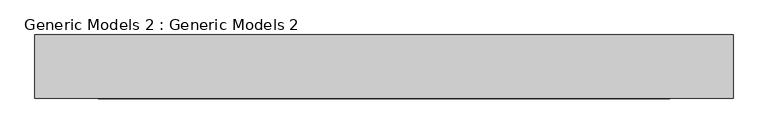
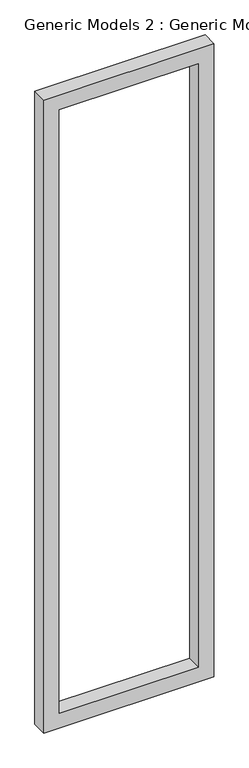
"""IFC4 building model written with IfcOpenShell, lengths in millimetres: proxy geometry, Generic Models 2 : Generic Models 2."""

from ifc_helpers import new_model, si_unit, frame, origin, place, context, project, spatial, polyline, outline, extrude, source, transform, mapped, element, save


def generic_models_2_generic_models_2_a6d57641(model_context):
    return source(origin(), model_context, "Body", "SweptSolid", [
        extrude(outline(polyline([(7672.7640825, -12487.4023867), (7672.7640825, -14163.8023867), (1077.9220303, -14163.8023867), (1077.9220303, -12487.4023867), (7672.7640825, -12487.4023867)]), holes=[polyline([(1230.3220303, -12639.8023867), (1230.3220303, -14011.4023867), (7520.3640825, -14011.4023867), (7520.3640825, -12639.8023867), (1230.3220303, -12639.8023867)])]), frame((0.0, -3137.7499863, 0.0), z_axis=(0.0, 1.0, 0.0), x_axis=(0.0, 0.0, 1.0)), (0.0, 0.0, 1.0), 152.4),
    ])


if __name__ == "__main__":
    model = new_model("IFC4")
    model_context = context("Model", 3, world=origin())
    ifc_project = project(units=[si_unit("LENGTHUNIT", "METRE", prefix="MILLI")], contexts=[model_context])
    site = spatial("IfcSite", under=ifc_project)
    building = spatial("IfcBuilding", under=site)
    placement = place(None, origin())
    generic_models_2_generic_models_2_shape = generic_models_2_generic_models_2_a6d57641(model_context)
    element("IfcBuildingElementProxy", 1, Name="Generic Models 2 : Generic Models 2", ObjectType="Generic Models 2 : Generic Models 2", at=placement, inside=building, context=model_context, shape_type="MappedRepresentation", body=[
        mapped(generic_models_2_generic_models_2_shape, transform((0.0, 0.0, 0.0), x_axis=(1.0, 0.0, 0.0), y_axis=(0.0, 1.0, 0.0), z_axis=(0.0, 0.0, 1.0))),
    ])
    save(model, "model.ifc")

# Revit data of these elements
# Element 1 (IfcBuildingElementProxy, "Generic Models 2 : Generic Models 2")
#   Materials on its faces: "accent wall"
# Materials
#   "accent wall": class "Generic", colour RGB 120 120 120, transparency 0, Cost = 0
